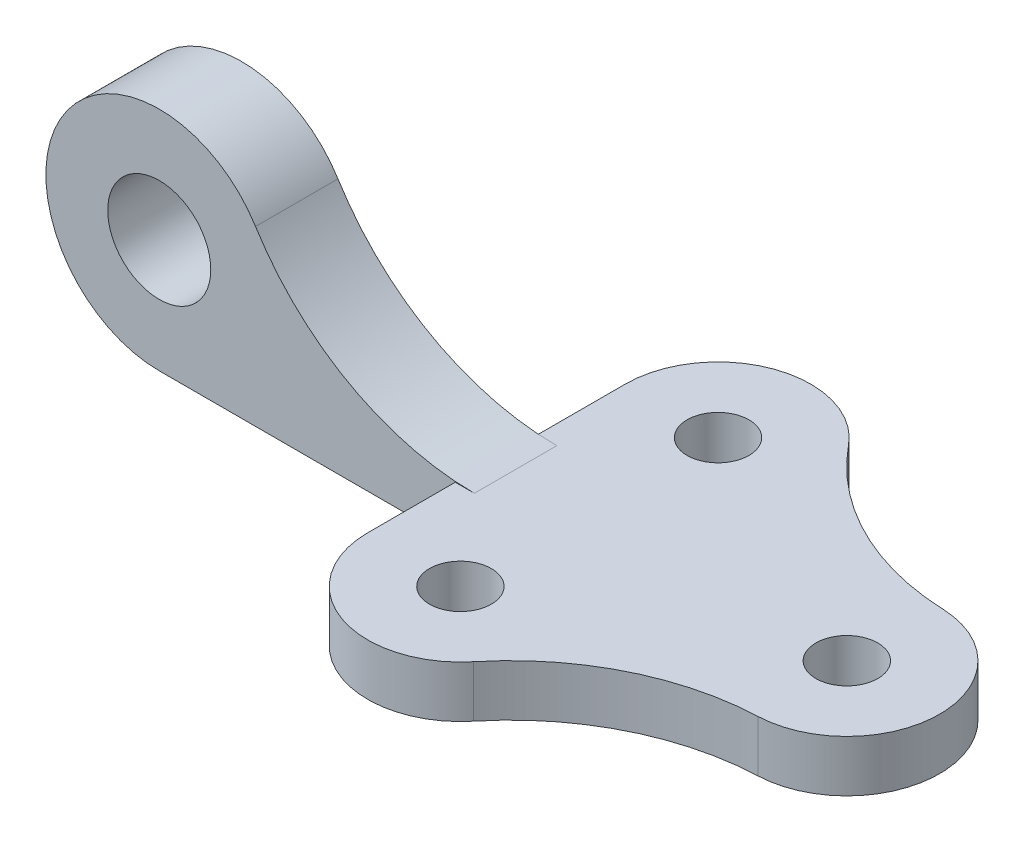
ISO-10303-21;
HEADER;
FILE_DESCRIPTION(('STEP AP214'),'2;1');
FILE_NAME('part.step','',(''),(''),'','','');
FILE_SCHEMA(('AUTOMOTIVE_DESIGN { 1 0 10303 214 1 1 1 1 }'));
ENDSEC;
DATA;
#1=APPLICATION_CONTEXT('core data for automotive mechanical design processes');
#2=APPLICATION_PROTOCOL_DEFINITION('international standard','automotive_design',2000,#1);
#3=PRODUCT_CONTEXT('',#1,'mechanical');
#4=PRODUCT('Part','Part','',(#3));
#5=PRODUCT_RELATED_PRODUCT_CATEGORY('part','',(#4));
#6=PRODUCT_DEFINITION_FORMATION('','',#4);
#7=PRODUCT_DEFINITION_CONTEXT('part definition',#1,'design');
#8=PRODUCT_DEFINITION('design','',#6,#7);
#9=PRODUCT_DEFINITION_SHAPE('','',#8);
#10=(LENGTH_UNIT() NAMED_UNIT(*) SI_UNIT(.MILLI.,.METRE.));
#11=(NAMED_UNIT(*) PLANE_ANGLE_UNIT() SI_UNIT($,.RADIAN.));
#12=(NAMED_UNIT(*) SI_UNIT($,.STERADIAN.) SOLID_ANGLE_UNIT());
#13=UNCERTAINTY_MEASURE_WITH_UNIT(LENGTH_MEASURE(1.E-05),#10,'distance_accuracy_value','');
#14=(GEOMETRIC_REPRESENTATION_CONTEXT(3) GLOBAL_UNCERTAINTY_ASSIGNED_CONTEXT((#13)) GLOBAL_UNIT_ASSIGNED_CONTEXT((#10,
#11,#12)) REPRESENTATION_CONTEXT('',''));
#15=CARTESIAN_POINT('',(0.,0.,0.));
#16=DIRECTION('',(0.,0.,1.));
#17=DIRECTION('',(1.,0.,0.));
#18=AXIS2_PLACEMENT_3D('',#15,#16,#17);
#19=CARTESIAN_POINT('',(-41.,22.,8.));
#20=DIRECTION('',(0.,0.,-1.));
#21=DIRECTION('',(-1.,0.,0.));
#22=AXIS2_PLACEMENT_3D('',#19,#20,#21);
#23=CYLINDRICAL_SURFACE('',#22,10.);
#24=CARTESIAN_POINT('',(-41.,22.,8.));
#25=DIRECTION('',(0.,0.,1.));
#26=DIRECTION('',(1.,0.,0.));
#27=AXIS2_PLACEMENT_3D('',#24,#25,#26);
#28=CIRCLE('',#27,10.);
#29=CARTESIAN_POINT('',(-31.,22.,8.));
#30=VERTEX_POINT('',#29);
#31=EDGE_CURVE('E237',#30,#30,#28,.T.);
#32=ORIENTED_EDGE('',*,*,#31,.T.);
#33=EDGE_LOOP('',(#32));
#34=FACE_BOUND('',#33,.T.);
#35=CARTESIAN_POINT('',(-41.,22.,-8.));
#36=DIRECTION('',(0.,0.,1.));
#37=DIRECTION('',(1.,0.,0.));
#38=AXIS2_PLACEMENT_3D('',#35,#36,#37);
#39=CIRCLE('',#38,10.);
#40=CARTESIAN_POINT('',(-31.,22.,-8.));
#41=VERTEX_POINT('',#40);
#42=EDGE_CURVE('E235',#41,#41,#39,.T.);
#43=ORIENTED_EDGE('',*,*,#42,.F.);
#44=EDGE_LOOP('',(#43));
#45=FACE_BOUND('',#44,.T.);
#46=ADVANCED_FACE('F66',(#34,#45),#23,.F.);
#47=CARTESIAN_POINT('',(-41.,22.,8.));
#48=DIRECTION('',(0.,0.,-1.));
#49=DIRECTION('',(-1.,0.,0.));
#50=AXIS2_PLACEMENT_3D('',#47,#48,#49);
#51=CYLINDRICAL_SURFACE('',#50,22.);
#52=CARTESIAN_POINT('',(-41.,22.,-8.));
#53=DIRECTION('',(0.,0.,1.));
#54=DIRECTION('',(1.,0.,0.));
#55=AXIS2_PLACEMENT_3D('',#52,#53,#54);
#56=CIRCLE('',#55,22.);
#57=CARTESIAN_POINT('',(-22.313585181597,33.6111111111111,-8.));
#58=VERTEX_POINT('',#57);
#59=CARTESIAN_POINT('',(-41.,0.,-8.));
#60=VERTEX_POINT('',#59);
#61=EDGE_CURVE('E244',#58,#60,#56,.T.);
#62=ORIENTED_EDGE('',*,*,#61,.T.);
#63=DIRECTION('',(0.,0.,-1.));
#64=VECTOR('',#63,1.);
#65=CARTESIAN_POINT('',(-41.,0.,8.));
#66=LINE('',#65,#64);
#67=CARTESIAN_POINT('',(-41.,0.,8.));
#68=VERTEX_POINT('',#67);
#69=EDGE_CURVE('E249',#68,#60,#66,.T.);
#70=ORIENTED_EDGE('',*,*,#69,.F.);
#71=CARTESIAN_POINT('',(-41.,22.,8.));
#72=DIRECTION('',(0.,0.,1.));
#73=DIRECTION('',(1.,0.,0.));
#74=AXIS2_PLACEMENT_3D('',#71,#72,#73);
#75=CIRCLE('',#74,22.);
#76=CARTESIAN_POINT('',(-22.313585181597,33.6111111111111,8.));
#77=VERTEX_POINT('',#76);
#78=EDGE_CURVE('E84',#77,#68,#75,.T.);
#79=ORIENTED_EDGE('',*,*,#78,.F.);
#80=DIRECTION('',(0.,0.,-1.));
#81=VECTOR('',#80,1.);
#82=CARTESIAN_POINT('',(-22.313585181597,33.6111111111111,8.));
#83=LINE('',#82,#81);
#84=EDGE_CURVE('E79',#77,#58,#83,.T.);
#85=ORIENTED_EDGE('',*,*,#84,.T.);
#86=EDGE_LOOP('',(#62,#70,#79,#85));
#87=FACE_BOUND('',#86,.T.);
#88=ADVANCED_FACE('F278',(#87),#51,.T.);
#89=CARTESIAN_POINT('',(0.,0.,8.));
#90=DIRECTION('',(0.,1.,0.));
#91=DIRECTION('',(0.,0.,1.));
#92=AXIS2_PLACEMENT_3D('',#89,#90,#91);
#93=PLANE('',#92);
#94=DIRECTION('',(1.,0.,0.));
#95=VECTOR('',#94,1.);
#96=CARTESIAN_POINT('',(0.,0.,-8.));
#97=LINE('',#96,#95);
#98=CARTESIAN_POINT('',(16.4455394056826,0.,-8.));
#99=VERTEX_POINT('',#98);
#100=EDGE_CURVE('E245',#60,#99,#97,.T.);
#101=ORIENTED_EDGE('',*,*,#100,.T.);
#102=DIRECTION('',(0.,0.,1.));
#103=VECTOR('',#102,1.);
#104=CARTESIAN_POINT('',(16.4455394056826,0.,-25.));
#105=LINE('',#104,#103);
#106=CARTESIAN_POINT('',(16.4455394056826,0.,-25.));
#107=VERTEX_POINT('',#106);
#108=EDGE_CURVE('E178',#107,#99,#105,.T.);
#109=ORIENTED_EDGE('',*,*,#108,.F.);
#110=CARTESIAN_POINT('',(34.4455394056826,0.,-25.));
#111=DIRECTION('',(0.,1.,0.));
#112=DIRECTION('',(0.,0.,1.));
#113=AXIS2_PLACEMENT_3D('',#110,#111,#112);
#114=CIRCLE('',#113,18.);
#115=CARTESIAN_POINT('',(48.4015573226198,0.,-36.3679181868155));
#116=VERTEX_POINT('',#115);
#117=EDGE_CURVE('E160',#116,#107,#114,.T.);
#118=ORIENTED_EDGE('',*,*,#117,.F.);
#119=CARTESIAN_POINT('',(87.1682737585563,0.,-67.9454687057473));
#120=DIRECTION('',(0.,-1.,0.));
#121=DIRECTION('',(0.,0.,1.));
#122=AXIS2_PLACEMENT_3D('',#119,#120,#121);
#123=CIRCLE('',#122,50.);
#124=CARTESIAN_POINT('',(85.1662632049727,0.,-17.985565245639));
#125=VERTEX_POINT('',#124);
#126=EDGE_CURVE('E175',#125,#116,#123,.T.);
#127=ORIENTED_EDGE('',*,*,#126,.F.);
#128=CARTESIAN_POINT('',(84.4455394056826,0.,0.));
#129=DIRECTION('',(0.,1.,0.));
#130=DIRECTION('',(0.,0.,1.));
#131=AXIS2_PLACEMENT_3D('',#128,#129,#130);
#132=CIRCLE('',#131,18.);
#133=CARTESIAN_POINT('',(85.1662632049727,0.,17.985565245639));
#134=VERTEX_POINT('',#133);
#135=EDGE_CURVE('E164',#134,#125,#132,.T.);
#136=ORIENTED_EDGE('',*,*,#135,.F.);
#137=CARTESIAN_POINT('',(87.1682737585563,0.,67.9454687057473));
#138=DIRECTION('',(0.,-1.,0.));
#139=DIRECTION('',(0.,0.,-1.));
#140=AXIS2_PLACEMENT_3D('',#137,#138,#139);
#141=CIRCLE('',#140,50.);
#142=CARTESIAN_POINT('',(48.4015573226197,0.,36.3679181868155));
#143=VERTEX_POINT('',#142);
#144=EDGE_CURVE('E192',#143,#134,#141,.T.);
#145=ORIENTED_EDGE('',*,*,#144,.F.);
#146=CARTESIAN_POINT('',(34.4455394056826,0.,25.));
#147=DIRECTION('',(0.,1.,0.));
#148=DIRECTION('',(0.,0.,1.));
#149=AXIS2_PLACEMENT_3D('',#146,#147,#148);
#150=CIRCLE('',#149,18.);
#151=CARTESIAN_POINT('',(16.4455394056826,0.,25.));
#152=VERTEX_POINT('',#151);
#153=EDGE_CURVE('E193',#152,#143,#150,.T.);
#154=ORIENTED_EDGE('',*,*,#153,.F.);
#155=CARTESIAN_POINT('',(16.4455394056826,0.,8.));
#156=VERTEX_POINT('',#155);
#157=EDGE_CURVE('E180',#156,#152,#105,.T.);
#158=ORIENTED_EDGE('',*,*,#157,.F.);
#159=DIRECTION('',(1.,0.,0.));
#160=VECTOR('',#159,1.);
#161=CARTESIAN_POINT('',(0.,0.,8.));
#162=LINE('',#161,#160);
#163=EDGE_CURVE('E232',#68,#156,#162,.T.);
#164=ORIENTED_EDGE('',*,*,#163,.F.);
#165=ORIENTED_EDGE('',*,*,#69,.T.);
#166=EDGE_LOOP('',(#101,#109,#118,#127,#136,#145,#154,#158,#164,#165));
#167=FACE_BOUND('',#166,.T.);
#168=CARTESIAN_POINT('',(84.4455394056826,0.,0.));
#169=DIRECTION('',(0.,1.,0.));
#170=DIRECTION('',(0.,0.,1.));
#171=AXIS2_PLACEMENT_3D('',#168,#169,#170);
#172=CIRCLE('',#171,6.);
#173=CARTESIAN_POINT('',(84.4455394056826,0.,6.));
#174=VERTEX_POINT('',#173);
#175=EDGE_CURVE('E199',#174,#174,#172,.T.);
#176=ORIENTED_EDGE('',*,*,#175,.T.);
#177=EDGE_LOOP('',(#176));
#178=FACE_BOUND('',#177,.T.);
#179=CARTESIAN_POINT('',(34.4455394056826,0.,25.));
#180=DIRECTION('',(0.,1.,0.));
#181=DIRECTION('',(0.,0.,1.));
#182=AXIS2_PLACEMENT_3D('',#179,#180,#181);
#183=CIRCLE('',#182,5.99999999999999);
#184=CARTESIAN_POINT('',(34.4455394056826,0.,31.));
#185=VERTEX_POINT('',#184);
#186=EDGE_CURVE('E313',#185,#185,#183,.T.);
#187=ORIENTED_EDGE('',*,*,#186,.T.);
#188=EDGE_LOOP('',(#187));
#189=FACE_BOUND('',#188,.T.);
#190=CARTESIAN_POINT('',(34.4455394056826,0.,-25.));
#191=DIRECTION('',(0.,1.,0.));
#192=DIRECTION('',(0.,0.,1.));
#193=AXIS2_PLACEMENT_3D('',#190,#191,#192);
#194=CIRCLE('',#193,5.99999999999999);
#195=CARTESIAN_POINT('',(34.4455394056826,0.,-19.));
#196=VERTEX_POINT('',#195);
#197=EDGE_CURVE('E301',#196,#196,#194,.T.);
#198=ORIENTED_EDGE('',*,*,#197,.T.);
#199=EDGE_LOOP('',(#198));
#200=FACE_BOUND('',#199,.T.);
#201=ADVANCED_FACE('F173',(#167,#178,#189,#200),#93,.F.);
#202=CARTESIAN_POINT('',(20.1555394056826,60.,8.));
#203=DIRECTION('',(0.,0.,-1.));
#204=DIRECTION('',(-1.,0.,0.));
#205=AXIS2_PLACEMENT_3D('',#202,#203,#204);
#206=CYLINDRICAL_SURFACE('',#205,50.);
#207=CARTESIAN_POINT('',(20.1555394056826,60.,-8.));
#208=DIRECTION('',(0.,0.,1.));
#209=DIRECTION('',(1.,0.,0.));
#210=AXIS2_PLACEMENT_3D('',#207,#208,#209);
#211=CIRCLE('',#210,50.);
#212=CARTESIAN_POINT('',(20.1555394056826,10.,-8.));
#213=VERTEX_POINT('',#212);
#214=EDGE_CURVE('E227',#58,#213,#211,.T.);
#215=ORIENTED_EDGE('',*,*,#214,.F.);
#216=ORIENTED_EDGE('',*,*,#84,.F.);
#217=CARTESIAN_POINT('',(20.1555394056826,60.,8.));
#218=DIRECTION('',(0.,0.,1.));
#219=DIRECTION('',(1.,0.,0.));
#220=AXIS2_PLACEMENT_3D('',#217,#218,#219);
#221=CIRCLE('',#220,50.);
#222=CARTESIAN_POINT('',(20.1555394056826,10.,8.));
#223=VERTEX_POINT('',#222);
#224=EDGE_CURVE('E230',#77,#223,#221,.T.);
#225=ORIENTED_EDGE('',*,*,#224,.T.);
#226=DIRECTION('',(0.,0.,-1.));
#227=VECTOR('',#226,1.);
#228=CARTESIAN_POINT('',(20.1555394056826,10.,8.));
#229=LINE('',#228,#227);
#230=EDGE_CURVE('E239',#223,#213,#229,.T.);
#231=ORIENTED_EDGE('',*,*,#230,.T.);
#232=EDGE_LOOP('',(#215,#216,#225,#231));
#233=FACE_BOUND('',#232,.T.);
#234=ADVANCED_FACE('F276',(#233),#206,.F.);
#235=CARTESIAN_POINT('',(0.,0.,-8.));
#236=DIRECTION('',(0.,0.,1.));
#237=DIRECTION('',(1.,0.,0.));
#238=AXIS2_PLACEMENT_3D('',#235,#236,#237);
#239=PLANE('',#238);
#240=DIRECTION('',(-1.,0.,0.));
#241=VECTOR('',#240,1.);
#242=CARTESIAN_POINT('',(0.,10.,-8.));
#243=LINE('',#242,#241);
#244=CARTESIAN_POINT('',(16.4455394056826,10.,-8.));
#245=VERTEX_POINT('',#244);
#246=EDGE_CURVE('E215',#213,#245,#243,.T.);
#247=ORIENTED_EDGE('',*,*,#246,.T.);
#248=DIRECTION('',(0.,-1.,0.));
#249=VECTOR('',#248,1.);
#250=CARTESIAN_POINT('',(16.4455394056826,0.,-8.));
#251=LINE('',#250,#249);
#252=EDGE_CURVE('E224',#245,#99,#251,.T.);
#253=ORIENTED_EDGE('',*,*,#252,.T.);
#254=ORIENTED_EDGE('',*,*,#100,.F.);
#255=ORIENTED_EDGE('',*,*,#61,.F.);
#256=ORIENTED_EDGE('',*,*,#214,.T.);
#257=EDGE_LOOP('',(#247,#253,#254,#255,#256));
#258=FACE_BOUND('',#257,.T.);
#259=ORIENTED_EDGE('',*,*,#42,.T.);
#260=EDGE_LOOP('',(#259));
#261=FACE_BOUND('',#260,.T.);
#262=ADVANCED_FACE('F254',(#258,#261),#239,.F.);
#263=CARTESIAN_POINT('',(0.,0.,8.));
#264=DIRECTION('',(0.,0.,1.));
#265=DIRECTION('',(1.,0.,0.));
#266=AXIS2_PLACEMENT_3D('',#263,#264,#265);
#267=PLANE('',#266);
#268=DIRECTION('',(0.,-1.,0.));
#269=VECTOR('',#268,1.);
#270=CARTESIAN_POINT('',(16.4455394056826,0.,8.));
#271=LINE('',#270,#269);
#272=CARTESIAN_POINT('',(16.4455394056826,10.,8.));
#273=VERTEX_POINT('',#272);
#274=EDGE_CURVE('E12',#273,#156,#271,.T.);
#275=ORIENTED_EDGE('',*,*,#274,.F.);
#276=DIRECTION('',(-1.,0.,0.));
#277=VECTOR('',#276,1.);
#278=CARTESIAN_POINT('',(0.,10.,8.));
#279=LINE('',#278,#277);
#280=EDGE_CURVE('E222',#223,#273,#279,.T.);
#281=ORIENTED_EDGE('',*,*,#280,.F.);
#282=ORIENTED_EDGE('',*,*,#224,.F.);
#283=ORIENTED_EDGE('',*,*,#78,.T.);
#284=ORIENTED_EDGE('',*,*,#163,.T.);
#285=EDGE_LOOP('',(#275,#281,#282,#283,#284));
#286=FACE_BOUND('',#285,.T.);
#287=ORIENTED_EDGE('',*,*,#31,.F.);
#288=EDGE_LOOP('',(#287));
#289=FACE_BOUND('',#288,.T.);
#290=ADVANCED_FACE('F277',(#286,#289),#267,.T.);
#291=CARTESIAN_POINT('',(0.,10.,8.));
#292=DIRECTION('',(0.,1.,0.));
#293=DIRECTION('',(0.,0.,1.));
#294=AXIS2_PLACEMENT_3D('',#291,#292,#293);
#295=PLANE('',#294);
#296=CARTESIAN_POINT('',(84.4455394056826,10.,0.));
#297=DIRECTION('',(0.,1.,0.));
#298=DIRECTION('',(0.,0.,1.));
#299=AXIS2_PLACEMENT_3D('',#296,#297,#298);
#300=CIRCLE('',#299,6.);
#301=CARTESIAN_POINT('',(84.4455394056826,10.,6.));
#302=VERTEX_POINT('',#301);
#303=EDGE_CURVE('E189',#302,#302,#300,.T.);
#304=ORIENTED_EDGE('',*,*,#303,.F.);
#305=EDGE_LOOP('',(#304));
#306=FACE_BOUND('',#305,.T.);
#307=ORIENTED_EDGE('',*,*,#246,.F.);
#308=ORIENTED_EDGE('',*,*,#230,.F.);
#309=ORIENTED_EDGE('',*,*,#280,.T.);
#310=DIRECTION('',(0.,0.,1.));
#311=VECTOR('',#310,1.);
#312=CARTESIAN_POINT('',(16.4455394056826,10.,-25.));
#313=LINE('',#312,#311);
#314=CARTESIAN_POINT('',(16.4455394056826,10.,25.));
#315=VERTEX_POINT('',#314);
#316=EDGE_CURVE('E205',#273,#315,#313,.T.);
#317=ORIENTED_EDGE('',*,*,#316,.T.);
#318=CARTESIAN_POINT('',(34.4455394056826,10.,25.));
#319=DIRECTION('',(0.,1.,0.));
#320=DIRECTION('',(0.,0.,1.));
#321=AXIS2_PLACEMENT_3D('',#318,#319,#320);
#322=CIRCLE('',#321,18.);
#323=CARTESIAN_POINT('',(48.4015573226197,10.,36.3679181868155));
#324=VERTEX_POINT('',#323);
#325=EDGE_CURVE('E206',#315,#324,#322,.T.);
#326=ORIENTED_EDGE('',*,*,#325,.T.);
#327=CARTESIAN_POINT('',(87.1682737585563,10.,67.9454687057473));
#328=DIRECTION('',(0.,-1.,0.));
#329=DIRECTION('',(0.,0.,-1.));
#330=AXIS2_PLACEMENT_3D('',#327,#328,#329);
#331=CIRCLE('',#330,50.);
#332=CARTESIAN_POINT('',(85.1662632049727,10.,17.985565245639));
#333=VERTEX_POINT('',#332);
#334=EDGE_CURVE('E184',#324,#333,#331,.T.);
#335=ORIENTED_EDGE('',*,*,#334,.T.);
#336=CARTESIAN_POINT('',(84.4455394056826,10.,0.));
#337=DIRECTION('',(0.,1.,0.));
#338=DIRECTION('',(0.,0.,1.));
#339=AXIS2_PLACEMENT_3D('',#336,#337,#338);
#340=CIRCLE('',#339,18.);
#341=CARTESIAN_POINT('',(85.1662632049727,10.,-17.985565245639));
#342=VERTEX_POINT('',#341);
#343=EDGE_CURVE('E182',#333,#342,#340,.T.);
#344=ORIENTED_EDGE('',*,*,#343,.T.);
#345=CARTESIAN_POINT('',(87.1682737585563,10.,-67.9454687057473));
#346=DIRECTION('',(0.,-1.,0.));
#347=DIRECTION('',(0.,0.,1.));
#348=AXIS2_PLACEMENT_3D('',#345,#346,#347);
#349=CIRCLE('',#348,50.);
#350=CARTESIAN_POINT('',(48.4015573226198,10.,-36.3679181868155));
#351=VERTEX_POINT('',#350);
#352=EDGE_CURVE('E196',#342,#351,#349,.T.);
#353=ORIENTED_EDGE('',*,*,#352,.T.);
#354=CARTESIAN_POINT('',(34.4455394056826,10.,-25.));
#355=DIRECTION('',(0.,1.,0.));
#356=DIRECTION('',(0.,0.,1.));
#357=AXIS2_PLACEMENT_3D('',#354,#355,#356);
#358=CIRCLE('',#357,18.);
#359=CARTESIAN_POINT('',(16.4455394056826,10.,-25.));
#360=VERTEX_POINT('',#359);
#361=EDGE_CURVE('E157',#351,#360,#358,.T.);
#362=ORIENTED_EDGE('',*,*,#361,.T.);
#363=EDGE_CURVE('E201',#360,#245,#313,.T.);
#364=ORIENTED_EDGE('',*,*,#363,.T.);
#365=EDGE_LOOP('',(#307,#308,#309,#317,#326,#335,#344,#353,#362,#364));
#366=FACE_BOUND('',#365,.T.);
#367=CARTESIAN_POINT('',(34.4455394056826,10.,-25.));
#368=DIRECTION('',(0.,1.,0.));
#369=DIRECTION('',(0.,0.,1.));
#370=AXIS2_PLACEMENT_3D('',#367,#368,#369);
#371=CIRCLE('',#370,5.99999999999999);
#372=CARTESIAN_POINT('',(34.4455394056826,10.,-19.));
#373=VERTEX_POINT('',#372);
#374=EDGE_CURVE('E308',#373,#373,#371,.T.);
#375=ORIENTED_EDGE('',*,*,#374,.F.);
#376=EDGE_LOOP('',(#375));
#377=FACE_BOUND('',#376,.T.);
#378=CARTESIAN_POINT('',(34.4455394056826,10.,25.));
#379=DIRECTION('',(0.,1.,0.));
#380=DIRECTION('',(0.,0.,1.));
#381=AXIS2_PLACEMENT_3D('',#378,#379,#380);
#382=CIRCLE('',#381,5.99999999999999);
#383=CARTESIAN_POINT('',(34.4455394056826,10.,31.));
#384=VERTEX_POINT('',#383);
#385=EDGE_CURVE('E314',#384,#384,#382,.T.);
#386=ORIENTED_EDGE('',*,*,#385,.F.);
#387=EDGE_LOOP('',(#386));
#388=FACE_BOUND('',#387,.T.);
#389=ADVANCED_FACE('F69',(#306,#366,#377,#388),#295,.T.);
#390=CARTESIAN_POINT('',(16.4455394056826,0.,-25.));
#391=DIRECTION('',(-1.,0.,0.));
#392=DIRECTION('',(0.,0.,1.));
#393=AXIS2_PLACEMENT_3D('',#390,#391,#392);
#394=PLANE('',#393);
#395=ORIENTED_EDGE('',*,*,#252,.F.);
#396=ORIENTED_EDGE('',*,*,#363,.F.);
#397=DIRECTION('',(0.,1.,0.));
#398=VECTOR('',#397,1.);
#399=CARTESIAN_POINT('',(16.4455394056826,0.,-25.));
#400=LINE('',#399,#398);
#401=EDGE_CURVE('E163',#107,#360,#400,.T.);
#402=ORIENTED_EDGE('',*,*,#401,.F.);
#403=ORIENTED_EDGE('',*,*,#108,.T.);
#404=EDGE_LOOP('',(#395,#396,#402,#403));
#405=FACE_BOUND('',#404,.T.);
#406=ADVANCED_FACE('F257',(#405),#394,.T.);
#407=CARTESIAN_POINT('',(87.1682737585563,0.,-67.9454687057473));
#408=DIRECTION('',(0.,1.,0.));
#409=DIRECTION('',(0.,0.,1.));
#410=AXIS2_PLACEMENT_3D('',#407,#408,#409);
#411=CYLINDRICAL_SURFACE('',#410,50.);
#412=ORIENTED_EDGE('',*,*,#352,.F.);
#413=DIRECTION('',(0.,1.,0.));
#414=VECTOR('',#413,1.);
#415=CARTESIAN_POINT('',(85.1662632049727,0.,-17.985565245639));
#416=LINE('',#415,#414);
#417=EDGE_CURVE('E179',#125,#342,#416,.T.);
#418=ORIENTED_EDGE('',*,*,#417,.F.);
#419=ORIENTED_EDGE('',*,*,#126,.T.);
#420=DIRECTION('',(0.,1.,0.));
#421=VECTOR('',#420,1.);
#422=CARTESIAN_POINT('',(48.4015573226198,0.,-36.3679181868155));
#423=LINE('',#422,#421);
#424=EDGE_CURVE('E152',#116,#351,#423,.T.);
#425=ORIENTED_EDGE('',*,*,#424,.T.);
#426=EDGE_LOOP('',(#412,#418,#419,#425));
#427=FACE_BOUND('',#426,.T.);
#428=ADVANCED_FACE('F177',(#427),#411,.F.);
#429=CARTESIAN_POINT('',(84.4455394056826,0.,0.));
#430=DIRECTION('',(0.,1.,0.));
#431=DIRECTION('',(0.,0.,1.));
#432=AXIS2_PLACEMENT_3D('',#429,#430,#431);
#433=CYLINDRICAL_SURFACE('',#432,18.);
#434=ORIENTED_EDGE('',*,*,#343,.F.);
#435=DIRECTION('',(0.,1.,0.));
#436=VECTOR('',#435,1.);
#437=CARTESIAN_POINT('',(85.1662632049727,0.,17.985565245639));
#438=LINE('',#437,#436);
#439=EDGE_CURVE('E213',#134,#333,#438,.T.);
#440=ORIENTED_EDGE('',*,*,#439,.F.);
#441=ORIENTED_EDGE('',*,*,#135,.T.);
#442=ORIENTED_EDGE('',*,*,#417,.T.);
#443=EDGE_LOOP('',(#434,#440,#441,#442));
#444=FACE_BOUND('',#443,.T.);
#445=ADVANCED_FACE('F270',(#444),#433,.T.);
#446=CARTESIAN_POINT('',(87.1682737585563,0.,67.9454687057473));
#447=DIRECTION('',(0.,1.,0.));
#448=DIRECTION('',(0.,0.,1.));
#449=AXIS2_PLACEMENT_3D('',#446,#447,#448);
#450=CYLINDRICAL_SURFACE('',#449,50.);
#451=ORIENTED_EDGE('',*,*,#334,.F.);
#452=DIRECTION('',(0.,1.,0.));
#453=VECTOR('',#452,1.);
#454=CARTESIAN_POINT('',(48.4015573226197,0.,36.3679181868155));
#455=LINE('',#454,#453);
#456=EDGE_CURVE('E214',#143,#324,#455,.T.);
#457=ORIENTED_EDGE('',*,*,#456,.F.);
#458=ORIENTED_EDGE('',*,*,#144,.T.);
#459=ORIENTED_EDGE('',*,*,#439,.T.);
#460=EDGE_LOOP('',(#451,#457,#458,#459));
#461=FACE_BOUND('',#460,.T.);
#462=ADVANCED_FACE('F337',(#461),#450,.F.);
#463=CARTESIAN_POINT('',(34.4455394056826,0.,25.));
#464=DIRECTION('',(0.,1.,0.));
#465=DIRECTION('',(0.,0.,1.));
#466=AXIS2_PLACEMENT_3D('',#463,#464,#465);
#467=CYLINDRICAL_SURFACE('',#466,18.);
#468=ORIENTED_EDGE('',*,*,#325,.F.);
#469=DIRECTION('',(0.,1.,0.));
#470=VECTOR('',#469,1.);
#471=CARTESIAN_POINT('',(16.4455394056826,0.,25.));
#472=LINE('',#471,#470);
#473=EDGE_CURVE('E220',#152,#315,#472,.T.);
#474=ORIENTED_EDGE('',*,*,#473,.F.);
#475=ORIENTED_EDGE('',*,*,#153,.T.);
#476=ORIENTED_EDGE('',*,*,#456,.T.);
#477=EDGE_LOOP('',(#468,#474,#475,#476));
#478=FACE_BOUND('',#477,.T.);
#479=ADVANCED_FACE('F273',(#478),#467,.T.);
#480=ORIENTED_EDGE('',*,*,#316,.F.);
#481=ORIENTED_EDGE('',*,*,#274,.T.);
#482=ORIENTED_EDGE('',*,*,#157,.T.);
#483=ORIENTED_EDGE('',*,*,#473,.T.);
#484=EDGE_LOOP('',(#480,#481,#482,#483));
#485=FACE_BOUND('',#484,.T.);
#486=ADVANCED_FACE('F274',(#485),#394,.T.);
#487=CARTESIAN_POINT('',(34.4455394056826,0.,-25.));
#488=DIRECTION('',(0.,1.,0.));
#489=DIRECTION('',(0.,0.,1.));
#490=AXIS2_PLACEMENT_3D('',#487,#488,#489);
#491=CYLINDRICAL_SURFACE('',#490,18.);
#492=ORIENTED_EDGE('',*,*,#361,.F.);
#493=ORIENTED_EDGE('',*,*,#424,.F.);
#494=ORIENTED_EDGE('',*,*,#117,.T.);
#495=ORIENTED_EDGE('',*,*,#401,.T.);
#496=EDGE_LOOP('',(#492,#493,#494,#495));
#497=FACE_BOUND('',#496,.T.);
#498=ADVANCED_FACE('F156',(#497),#491,.T.);
#499=CARTESIAN_POINT('',(84.4455394056826,0.,0.));
#500=DIRECTION('',(0.,1.,0.));
#501=DIRECTION('',(0.,0.,1.));
#502=AXIS2_PLACEMENT_3D('',#499,#500,#501);
#503=CYLINDRICAL_SURFACE('',#502,6.);
#504=ORIENTED_EDGE('',*,*,#303,.T.);
#505=EDGE_LOOP('',(#504));
#506=FACE_BOUND('',#505,.T.);
#507=ORIENTED_EDGE('',*,*,#175,.F.);
#508=EDGE_LOOP('',(#507));
#509=FACE_BOUND('',#508,.T.);
#510=ADVANCED_FACE('F332',(#506,#509),#503,.F.);
#511=CARTESIAN_POINT('',(34.4455394056826,0.,-25.));
#512=DIRECTION('',(0.,1.,0.));
#513=DIRECTION('',(0.,0.,1.));
#514=AXIS2_PLACEMENT_3D('',#511,#512,#513);
#515=CYLINDRICAL_SURFACE('',#514,5.99999999999999);
#516=ORIENTED_EDGE('',*,*,#197,.F.);
#517=EDGE_LOOP('',(#516));
#518=FACE_BOUND('',#517,.T.);
#519=ORIENTED_EDGE('',*,*,#374,.T.);
#520=EDGE_LOOP('',(#519));
#521=FACE_BOUND('',#520,.T.);
#522=ADVANCED_FACE('F322',(#518,#521),#515,.F.);
#523=CARTESIAN_POINT('',(34.4455394056826,0.,25.));
#524=DIRECTION('',(0.,1.,0.));
#525=DIRECTION('',(0.,0.,1.));
#526=AXIS2_PLACEMENT_3D('',#523,#524,#525);
#527=CYLINDRICAL_SURFACE('',#526,5.99999999999999);
#528=ORIENTED_EDGE('',*,*,#186,.F.);
#529=EDGE_LOOP('',(#528));
#530=FACE_BOUND('',#529,.T.);
#531=ORIENTED_EDGE('',*,*,#385,.T.);
#532=EDGE_LOOP('',(#531));
#533=FACE_BOUND('',#532,.T.);
#534=ADVANCED_FACE('F321',(#530,#533),#527,.F.);
#535=CLOSED_SHELL('',(#46,#88,#201,#234,#262,#290,#389,#406,#428,#445,#462,#479,#486,#498,#510,
#522,#534));
#536=MANIFOLD_SOLID_BREP('B2',#535);
#537=ADVANCED_BREP_SHAPE_REPRESENTATION('',(#18,#536),#14);
#538=SHAPE_DEFINITION_REPRESENTATION(#9,#537);
ENDSEC;
END-ISO-10303-21;
